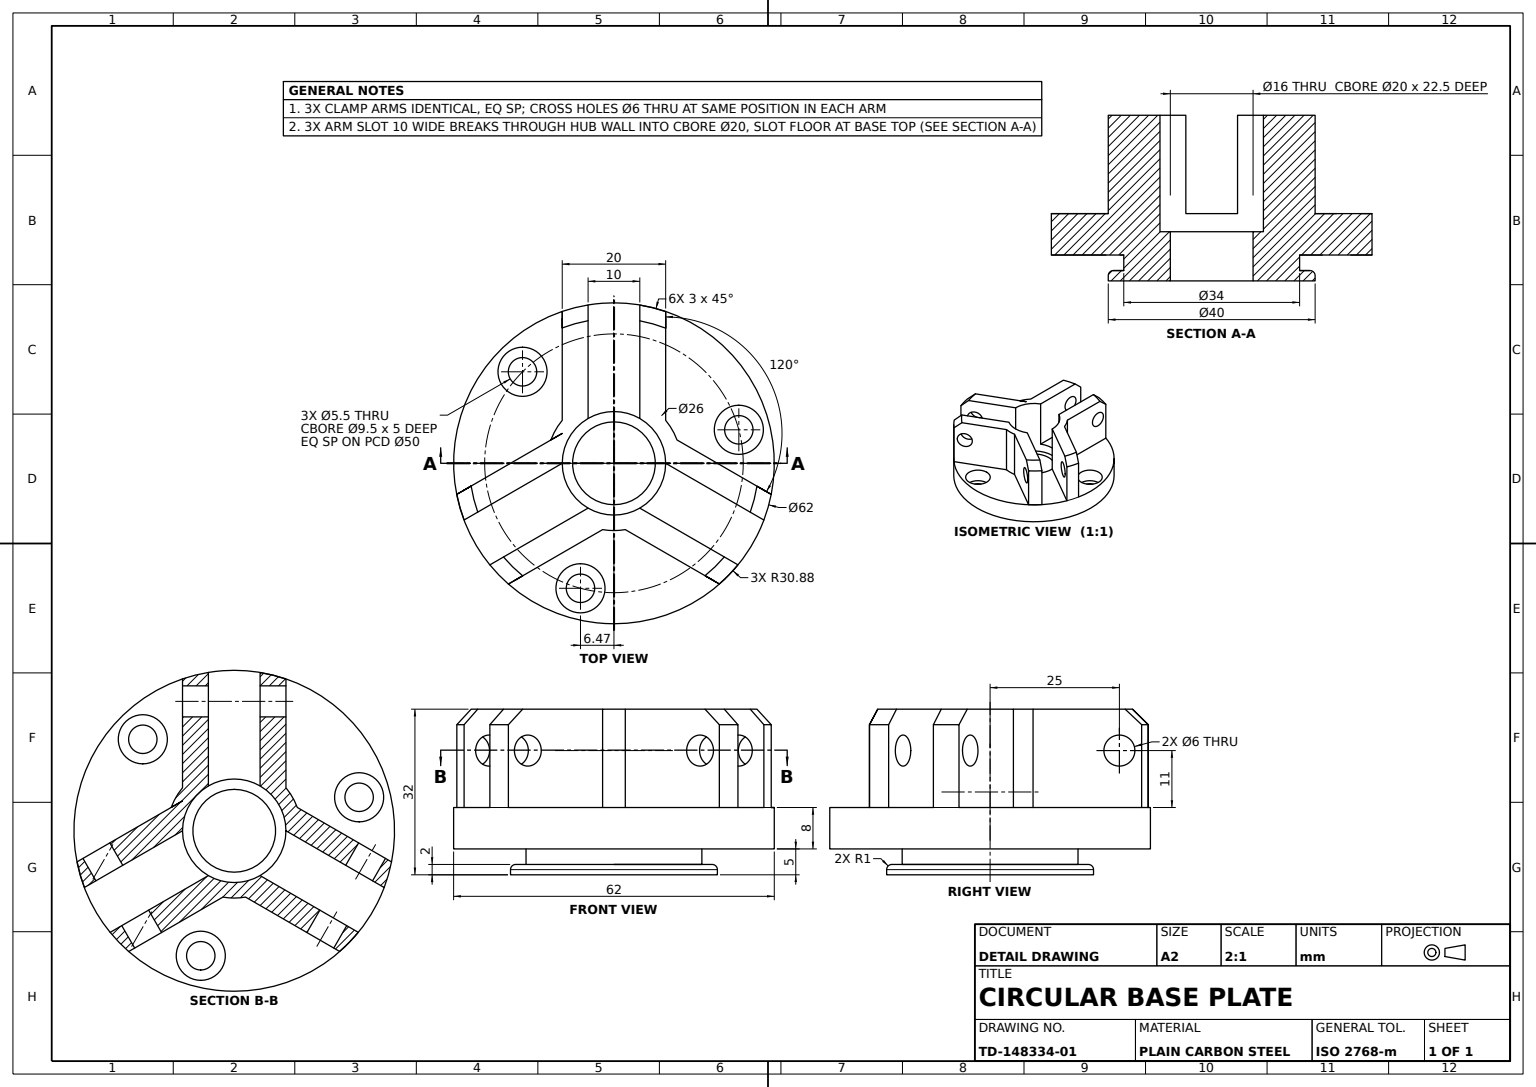
SolidWorks part; units mm, degrees
material "Plain Carbon Steel"
ref_plane "Front Plane" through (0, 0, 0) normal (0, 0, 1) x (1, 0, 0)
ref_plane "Top Plane" through (0, 0, 0) normal (0, 1, 0) x (1, 0, 0)
ref_plane "Right Plane" through (0, 0, 0) normal (1, 0, 0) x (0, 0, -1)
sketch "Base Disc Sketch" plane through (0, 0, 0) normal (0, 1, 0) x (1, 0, 0)
  circle A0 centre (0, 0) radius 31
  dimension "D1" = 62
extrude "Base Disc Ø62" add sketch "Base Disc Sketch" along normal blind 13
sketch "Clamp Arms Sketch" plane through (0, 13, 0) normal (0, 1, 0) x (1, 0, 0)
  line L2 (10, 29.3044) -> (10, 5.7735)
  line L4 (-10, 29.3428) -> (-10, 5.7735)
  line L6 (30.4116, -6.0111) -> (10, 5.7735)
  line L7 (5, 30.5709) -> (5, 2.8868)
  line L8 (-5, 30.5893) -> (-5, 2.8868)
  line L9 (28.9911, -10.9645) -> (5, 2.8868)
  line L10 (23.9752, -19.6156) -> (0, -5.7735)
  line L11 (20.3783, -23.3124) -> (0, -11.547)
  line L12 (-20.4116, -23.3317) -> (0, -11.547)
  line L13 (-23.9911, -19.6248) -> (0, -5.7735)
  line L14 (-28.9752, -10.9553) -> (-5, 2.8868)
  line L15 (-30.3783, -5.9919) -> (-10, 5.7735)
  circle A0 centre (0, 0) radius 31 construction
  arc A2 (30.4116, -6.0111) -> (28.9911, -10.9645) centre (0.1211, -0.0051) cw
  arc A3 (-10, 29.3428) -> (-5, 30.5893) centre (-0.0561, 0.1074) cw
  arc A4 (-20.4116, -23.3317) -> (-23.9911, -19.6248) centre (-0.065, -0.1023) cw
  arc A5 (5, 30.5709) -> (10, 29.3044) centre (-0.0561, 0.1074) cw
  arc A6 (23.9752, -19.6156) -> (20.3783, -23.3124) centre (0.1211, -0.0051) cw
  arc A7 (-28.9752, -10.9553) -> (-30.3783, -5.9919) centre (-0.065, -0.1023) cw
  dimension "D1" = 3
  dimension "D3" = 30.8802
  dimension "D4" = 0.1211
  dimension "D5" = 5
  dimension "D6" = 10
  dimension "D7" = 20.3783
  dimension "D8" = 28.9911
  dimension "D9" = 0.0561
  dimension "D10" = 0.065
  dimension "D2" = 3
extrude "Clamp Arms" add sketch "Clamp Arms Sketch" along normal blind 19
sketch "Centre Bore Sketch" plane through (0, 32, 0) normal (0, 1, 0) x (1, 0, 0)
  circle A0 centre (0, 0) radius 10
  dimension "D1" = 20
extrude "Centre Bore" cut sketch "Centre Bore Sketch" against normal blind 22.5
sketch "Centre Hub Sketch" plane through (0, 32, 0) normal (0, 1, 0) x (1, 0, 0)
  line L0 (-10, 8.3066) -> (-10, 5.7735)
  line L1 (-10, 29.3428) -> (-10, 5.7735) construction
  line L2 (-10, 5.7735) -> (-12.1883, 4.5216)
  line L3 (10, 8.3066) -> (10, 5.7735)
  line L4 (10, 5.7735) -> (10, 29.3044) construction
  line L5 (10, 5.7735) -> (12.1937, 4.5069)
  line L6 (30.4116, -6.0111) -> (10, 5.7735) construction
  line L7 (-2.1937, -12.8136) -> (0, -11.547)
  line L8 (-20.4116, -23.3317) -> (0, -11.547) construction
  line L9 (0, -11.547) -> (2.1937, -12.8136)
  line L10 (0, -11.547) -> (20.3783, -23.3124) construction
  arc A0 (12.1937, 4.5069) -> (10, 8.3066) centre (0, 0) ccw
  arc A1 (-2.1937, -12.8136) -> (2.1937, -12.8136) centre (0, 0) ccw
  arc A2 (-10, 8.3066) -> (-12.1883, 4.5216) centre (0, 0) ccw
  dimension "D1" = 13
  dimension "D2" = 2.1883
extrude "Centre Hub" add sketch "Centre Hub Sketch" against normal blind 20
sketch "Mounting Counterbores Sketch" plane through (0, 13, 0) normal (0, 1, 0) x (1, 0, 0)
  line L0 (-10, 29.3429) -> (-10, 8.3066) construction
  arc A0 (-20.7022, 14.015) -> (-10.9211, -22.4884) centre (0, 0) ccw
  circle A1 centre (-6.4705, -24.1481) radius 4.75
  circle A2 centre (-17.6777, 17.6777) radius 4.75
  circle A3 centre (24.1481, 6.4705) radius 4.75
  arc A4 (22.4884, 10.9211) -> (-14.015, 20.7022) centre (0, 0) ccw
  arc A5 (-1.7863, -24.9361) -> (24.9361, 1.7863) centre (0, 0) ccw
  dimension "D1" = 3
  dimension "D2" = 9.5
  dimension "D3" = 3.5295
  dimension "D5" = 25
extrude "Mounting Counterbores" cut sketch "Mounting Counterbores Sketch" against normal blind 5 contours A1 | A3 | A2
sketch "Arm Cross Hole 1 Sketch" plane through (-10, 0, 0) normal (-1, 0, 0) x (0, 0, 1)
  line L0 (-29.3429, 13) -> (-8.3066, 13) construction
  circle A0 centre (-25, 24) radius 3
  dimension "D1" = 6
  dimension "D2" = 4.3429
  dimension "D3" = 11
extrude "Arm Cross Hole 1" cut sketch "Arm Cross Hole 1 Sketch" against normal blind 32
sketch "Arm Cross Hole 2 Sketch" plane through (5, 0, -8.6603) normal (0.5, 0, -0.866) x (-0.866, 0, -0.5)
  line L0 (-8.3066, 13) -> (-8.3066, 32) construction
  line L1 (-29.3428, 13) -> (-8.3066, 13) construction
  circle A0 centre (-25, 24) radius 3
  dimension "D1" = 6
  dimension "D2" = 16.6934
  dimension "D3" = 11
extrude "Arm Cross Hole 2" cut sketch "Arm Cross Hole 2 Sketch" against normal blind 32
sketch "Arm Cross Hole 3 Sketch" plane through (5, 0, 8.6603) normal (0.5, 0, 0.866) x (0.866, 0, -0.5)
  line L0 (-8.3066, 13) -> (-8.3066, 32) construction
  line L1 (-29.343, 13) -> (-8.3066, 13) construction
  circle A0 centre (-25, 24) radius 3
  dimension "D1" = 6
  dimension "D2" = 16.6934
  dimension "D3" = 11
extrude "Arm Cross Hole 3" cut sketch "Arm Cross Hole 3 Sketch" against normal blind 32
sketch "Mounting Holes Sketch" plane through (0, 8, 0) normal (0, 1, 0) x (1, 0, 0)
  circle A0 centre (-17.6777, 17.6777) radius 2.75
  circle A1 centre (24.1481, 6.4705) radius 2.75
  circle A2 centre (-6.4705, -24.1481) radius 2.75
  dimension "D1" = 5.5
extrude "Mounting Holes 3x" cut sketch "Mounting Holes Sketch" against normal blind 32
sketch "Centre Through Bore Sketch" plane through (0, 9.5, 0) normal (0, 1, 0) x (1, 0, 0)
  circle A0 centre (0, 0) radius 8
  dimension "D1" = 16
extrude "Centre Through Bore" cut sketch "Centre Through Bore Sketch" against normal blind 32
chamfer "Arm Chamfer 1" distance 3 angle 45 1 edges at (-29.7806, 32, 8.503)
chamfer "Arm Chamfer 2" distance 3 angle 45 1 edges at (-22.2788, 32, 21.553)
chamfer "Arm Chamfer 3" distance 3 angle 45 1 edges at (22.2541, 32, 21.5392)
chamfer "Arm Chamfer 4" distance 3 angle 45 1 edges at (29.8049, 32, 8.5175)
chamfer "Arm Chamfer 5" distance 3 angle 45 1 edges at (7.5265, 32, -30.0422)
chamfer "Arm Chamfer 6" distance 3 angle 45 1 edges at (-7.526, 32, -30.0705)
sketch "Bottom Recess Sketch" plane through (0, 0, 0) normal (0, -1, 0) x (1, 0, 0)
  circle A0 centre (0, 0) radius 31
  dimension "D1" = 62
extrude "Bottom Recess" cut sketch "Bottom Recess Sketch" against normal blind 5
sketch "Recess Ring Sketch" plane through (0, 5, 0) normal (0, -1, 0) x (1, 0, 0)
  circle A0 centre (0, 0) radius 17
  dimension "D1" = 34
extrude "Recess Ring" add sketch "Recess Ring Sketch" along normal blind 3
sketch "Locating Lip Sketch" plane through (0, 2, 0) normal (0, -1, 0) x (1, 0, 0)
  circle A0 centre (0, 0) radius 20
  dimension "D1" = 40
extrude "Locating Lip" add sketch "Locating Lip Sketch" along normal blind 2
fillet "Locating Lip Fillet R1" radius 1 1 edges at (0, 2, -20)
sketch "Lip Bore Sketch" plane through (0, 5, 0) normal (0, 1, 0) x (1, 0, 0)
  circle A0 centre (0, 0) radius 8
  dimension "D1" = 16
extrude "Lip Bore" cut sketch "Lip Bore Sketch" against normal blind 19
